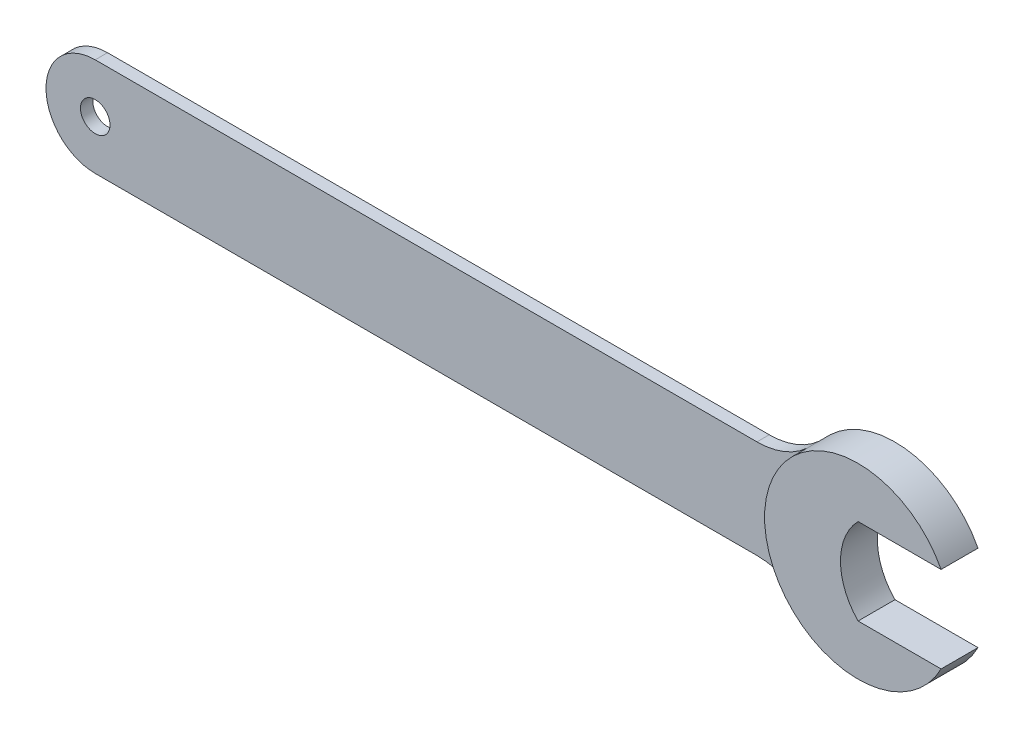
ISO-10303-21;
HEADER;
FILE_DESCRIPTION(('STEP AP214'),'2;1');
FILE_NAME('part.step','',(''),(''),'','','');
FILE_SCHEMA(('AUTOMOTIVE_DESIGN { 1 0 10303 214 1 1 1 1 }'));
ENDSEC;
DATA;
#1=APPLICATION_CONTEXT('core data for automotive mechanical design processes');
#2=APPLICATION_PROTOCOL_DEFINITION('international standard','automotive_design',2000,#1);
#3=PRODUCT_CONTEXT('',#1,'mechanical');
#4=PRODUCT('Part','Part','',(#3));
#5=PRODUCT_RELATED_PRODUCT_CATEGORY('part','',(#4));
#6=PRODUCT_DEFINITION_FORMATION('','',#4);
#7=PRODUCT_DEFINITION_CONTEXT('part definition',#1,'design');
#8=PRODUCT_DEFINITION('design','',#6,#7);
#9=PRODUCT_DEFINITION_SHAPE('','',#8);
#10=(LENGTH_UNIT() NAMED_UNIT(*) SI_UNIT(.MILLI.,.METRE.));
#11=(NAMED_UNIT(*) PLANE_ANGLE_UNIT() SI_UNIT($,.RADIAN.));
#12=(NAMED_UNIT(*) SI_UNIT($,.STERADIAN.) SOLID_ANGLE_UNIT());
#13=UNCERTAINTY_MEASURE_WITH_UNIT(LENGTH_MEASURE(1.E-05),#10,'distance_accuracy_value','');
#14=(GEOMETRIC_REPRESENTATION_CONTEXT(3) GLOBAL_UNCERTAINTY_ASSIGNED_CONTEXT((#13)) GLOBAL_UNIT_ASSIGNED_CONTEXT((#10,
#11,#12)) REPRESENTATION_CONTEXT('',''));
#15=CARTESIAN_POINT('',(0.,0.,0.));
#16=DIRECTION('',(0.,0.,1.));
#17=DIRECTION('',(1.,0.,0.));
#18=AXIS2_PLACEMENT_3D('',#15,#16,#17);
#19=CARTESIAN_POINT('',(315.,20.,0.));
#20=DIRECTION('',(0.,0.,1.));
#21=DIRECTION('',(1.,0.,0.));
#22=AXIS2_PLACEMENT_3D('',#19,#20,#21);
#23=CYLINDRICAL_SURFACE('',#22,38.);
#24=CARTESIAN_POINT('',(315.,20.,-5.));
#25=DIRECTION('',(0.,0.,-1.));
#26=DIRECTION('',(-1.,0.,0.));
#27=AXIS2_PLACEMENT_3D('',#24,#25,#26);
#28=CIRCLE('',#27,38.);
#29=CARTESIAN_POINT('',(348.730549951046,2.5,-5.));
#30=VERTEX_POINT('',#29);
#31=CARTESIAN_POINT('',(348.730549951046,37.5,-5.));
#32=VERTEX_POINT('',#31);
#33=EDGE_CURVE('E149',#30,#32,#28,.T.);
#34=ORIENTED_EDGE('',*,*,#33,.F.);
#35=DIRECTION('',(0.,0.,1.));
#36=VECTOR('',#35,1.);
#37=CARTESIAN_POINT('',(348.730549951046,2.5,0.));
#38=LINE('',#37,#36);
#39=CARTESIAN_POINT('',(348.730549951046,2.5,10.));
#40=VERTEX_POINT('',#39);
#41=EDGE_CURVE('E171',#30,#40,#38,.T.);
#42=ORIENTED_EDGE('',*,*,#41,.T.);
#43=CARTESIAN_POINT('',(315.,20.,10.));
#44=DIRECTION('',(0.,0.,1.));
#45=DIRECTION('',(1.,0.,0.));
#46=AXIS2_PLACEMENT_3D('',#43,#44,#45);
#47=CIRCLE('',#46,38.);
#48=CARTESIAN_POINT('',(348.730549951046,37.5,10.));
#49=VERTEX_POINT('',#48);
#50=EDGE_CURVE('E161',#49,#40,#47,.T.);
#51=ORIENTED_EDGE('',*,*,#50,.F.);
#52=DIRECTION('',(0.,0.,1.));
#53=VECTOR('',#52,1.);
#54=CARTESIAN_POINT('',(348.730549951046,37.5,0.));
#55=LINE('',#54,#53);
#56=EDGE_CURVE('E179',#32,#49,#55,.T.);
#57=ORIENTED_EDGE('',*,*,#56,.F.);
#58=EDGE_LOOP('',(#34,#42,#51,#57));
#59=FACE_BOUND('',#58,.T.);
#60=CARTESIAN_POINT('',(315.,20.,5.));
#61=DIRECTION('',(0.,0.,1.));
#62=DIRECTION('',(1.,0.,0.));
#63=AXIS2_PLACEMENT_3D('',#60,#61,#62);
#64=CIRCLE('',#63,38.);
#65=CARTESIAN_POINT('',(289.245570139499,47.9411764705883,5.));
#66=VERTEX_POINT('',#65);
#67=CARTESIAN_POINT('',(289.245570139499,-7.94117647058826,5.));
#68=VERTEX_POINT('',#67);
#69=EDGE_CURVE('E49',#66,#68,#64,.T.);
#70=ORIENTED_EDGE('',*,*,#69,.T.);
#71=DIRECTION('',(0.,0.,-1.));
#72=VECTOR('',#71,1.);
#73=CARTESIAN_POINT('',(289.245570139499,-7.94117647058827,5.));
#74=LINE('',#73,#72);
#75=CARTESIAN_POINT('',(289.245570139499,-7.94117647058827,0.));
#76=VERTEX_POINT('',#75);
#77=EDGE_CURVE('E130',#68,#76,#74,.T.);
#78=ORIENTED_EDGE('',*,*,#77,.T.);
#79=CARTESIAN_POINT('',(315.,20.,0.));
#80=DIRECTION('',(0.,0.,-1.));
#81=DIRECTION('',(-1.,0.,0.));
#82=AXIS2_PLACEMENT_3D('',#79,#80,#81);
#83=CIRCLE('',#82,38.);
#84=CARTESIAN_POINT('',(289.245570139499,47.9411764705882,0.));
#85=VERTEX_POINT('',#84);
#86=EDGE_CURVE('E11',#76,#85,#83,.T.);
#87=ORIENTED_EDGE('',*,*,#86,.T.);
#88=DIRECTION('',(0.,0.,-1.));
#89=VECTOR('',#88,1.);
#90=CARTESIAN_POINT('',(289.245570139499,47.9411764705883,5.));
#91=LINE('',#90,#89);
#92=EDGE_CURVE('E145',#66,#85,#91,.T.);
#93=ORIENTED_EDGE('',*,*,#92,.F.);
#94=EDGE_LOOP('',(#70,#78,#87,#93));
#95=FACE_BOUND('',#94,.T.);
#96=ADVANCED_FACE('F41',(#59,#95),#23,.T.);
#97=CARTESIAN_POINT('',(315.,40.,5.));
#98=DIRECTION('',(0.,-1.,0.));
#99=DIRECTION('',(0.,0.,-1.));
#100=AXIS2_PLACEMENT_3D('',#97,#98,#99);
#101=PLANE('',#100);
#102=DIRECTION('',(0.,0.,-1.));
#103=VECTOR('',#102,1.);
#104=CARTESIAN_POINT('',(268.913125512788,40.,5.));
#105=LINE('',#104,#103);
#106=CARTESIAN_POINT('',(268.913125512788,40.,5.));
#107=VERTEX_POINT('',#106);
#108=CARTESIAN_POINT('',(268.913125512788,40.,0.));
#109=VERTEX_POINT('',#108);
#110=EDGE_CURVE('E148',#107,#109,#105,.T.);
#111=ORIENTED_EDGE('',*,*,#110,.T.);
#112=DIRECTION('',(-1.,0.,0.));
#113=VECTOR('',#112,1.);
#114=CARTESIAN_POINT('',(315.,40.,0.));
#115=LINE('',#114,#113);
#116=CARTESIAN_POINT('',(0.,40.,0.));
#117=VERTEX_POINT('',#116);
#118=EDGE_CURVE('E192',#109,#117,#115,.T.);
#119=ORIENTED_EDGE('',*,*,#118,.T.);
#120=DIRECTION('',(0.,0.,-1.));
#121=VECTOR('',#120,1.);
#122=CARTESIAN_POINT('',(0.,40.,5.));
#123=LINE('',#122,#121);
#124=CARTESIAN_POINT('',(0.,40.,5.));
#125=VERTEX_POINT('',#124);
#126=EDGE_CURVE('E191',#125,#117,#123,.T.);
#127=ORIENTED_EDGE('',*,*,#126,.F.);
#128=DIRECTION('',(-1.,0.,0.));
#129=VECTOR('',#128,1.);
#130=CARTESIAN_POINT('',(315.,40.,5.));
#131=LINE('',#130,#129);
#132=EDGE_CURVE('E194',#107,#125,#131,.T.);
#133=ORIENTED_EDGE('',*,*,#132,.F.);
#134=EDGE_LOOP('',(#111,#119,#127,#133));
#135=FACE_BOUND('',#134,.T.);
#136=ADVANCED_FACE('F206',(#135),#101,.F.);
#137=CARTESIAN_POINT('',(0.,0.,0.));
#138=DIRECTION('',(0.,0.,1.));
#139=DIRECTION('',(1.,0.,0.));
#140=AXIS2_PLACEMENT_3D('',#137,#138,#139);
#141=PLANE('',#140);
#142=CARTESIAN_POINT('',(0.,20.,0.));
#143=DIRECTION('',(0.,0.,-1.));
#144=DIRECTION('',(-1.,0.,0.));
#145=AXIS2_PLACEMENT_3D('',#142,#143,#144);
#146=CIRCLE('',#145,6.);
#147=CARTESIAN_POINT('',(-6.,20.,0.));
#148=VERTEX_POINT('',#147);
#149=EDGE_CURVE('E139',#148,#148,#146,.T.);
#150=ORIENTED_EDGE('',*,*,#149,.F.);
#151=EDGE_LOOP('',(#150));
#152=FACE_BOUND('',#151,.T.);
#153=ORIENTED_EDGE('',*,*,#86,.F.);
#154=CARTESIAN_POINT('',(268.913125512788,-30.,0.));
#155=DIRECTION('',(0.,0.,1.));
#156=DIRECTION('',(1.,0.,0.));
#157=AXIS2_PLACEMENT_3D('',#154,#155,#156);
#158=CIRCLE('',#157,30.);
#159=CARTESIAN_POINT('',(268.913125512788,0.,0.));
#160=VERTEX_POINT('',#159);
#161=EDGE_CURVE('E118',#76,#160,#158,.T.);
#162=ORIENTED_EDGE('',*,*,#161,.T.);
#163=DIRECTION('',(1.,0.,0.));
#164=VECTOR('',#163,1.);
#165=CARTESIAN_POINT('',(0.,0.,0.));
#166=LINE('',#165,#164);
#167=CARTESIAN_POINT('',(0.,0.,0.));
#168=VERTEX_POINT('',#167);
#169=EDGE_CURVE('E59',#168,#160,#166,.T.);
#170=ORIENTED_EDGE('',*,*,#169,.F.);
#171=CARTESIAN_POINT('',(0.,20.,0.));
#172=DIRECTION('',(0.,0.,1.));
#173=DIRECTION('',(1.,0.,0.));
#174=AXIS2_PLACEMENT_3D('',#171,#172,#173);
#175=CIRCLE('',#174,20.);
#176=EDGE_CURVE('E183',#117,#168,#175,.T.);
#177=ORIENTED_EDGE('',*,*,#176,.F.);
#178=ORIENTED_EDGE('',*,*,#118,.F.);
#179=CARTESIAN_POINT('',(268.913125512788,70.,0.));
#180=DIRECTION('',(0.,0.,1.));
#181=DIRECTION('',(1.,0.,0.));
#182=AXIS2_PLACEMENT_3D('',#179,#180,#181);
#183=CIRCLE('',#182,30.);
#184=EDGE_CURVE('E124',#109,#85,#183,.T.);
#185=ORIENTED_EDGE('',*,*,#184,.T.);
#186=EDGE_LOOP('',(#153,#162,#170,#177,#178,#185));
#187=FACE_BOUND('',#186,.T.);
#188=ADVANCED_FACE('F120',(#152,#187),#141,.F.);
#189=CARTESIAN_POINT('',(0.,0.,5.));
#190=DIRECTION('',(0.,1.,0.));
#191=DIRECTION('',(0.,0.,1.));
#192=AXIS2_PLACEMENT_3D('',#189,#190,#191);
#193=PLANE('',#192);
#194=ORIENTED_EDGE('',*,*,#169,.T.);
#195=DIRECTION('',(0.,0.,-1.));
#196=VECTOR('',#195,1.);
#197=CARTESIAN_POINT('',(268.913125512788,0.,5.));
#198=LINE('',#197,#196);
#199=CARTESIAN_POINT('',(268.913125512788,0.,5.));
#200=VERTEX_POINT('',#199);
#201=EDGE_CURVE('E64',#200,#160,#198,.T.);
#202=ORIENTED_EDGE('',*,*,#201,.F.);
#203=DIRECTION('',(1.,0.,0.));
#204=VECTOR('',#203,1.);
#205=CARTESIAN_POINT('',(0.,0.,5.));
#206=LINE('',#205,#204);
#207=CARTESIAN_POINT('',(0.,0.,5.));
#208=VERTEX_POINT('',#207);
#209=EDGE_CURVE('E188',#208,#200,#206,.T.);
#210=ORIENTED_EDGE('',*,*,#209,.F.);
#211=DIRECTION('',(0.,0.,-1.));
#212=VECTOR('',#211,1.);
#213=CARTESIAN_POINT('',(0.,0.,5.));
#214=LINE('',#213,#212);
#215=EDGE_CURVE('E178',#208,#168,#214,.T.);
#216=ORIENTED_EDGE('',*,*,#215,.T.);
#217=EDGE_LOOP('',(#194,#202,#210,#216));
#218=FACE_BOUND('',#217,.T.);
#219=ADVANCED_FACE('F43',(#218),#193,.F.);
#220=CARTESIAN_POINT('',(0.,0.,5.));
#221=DIRECTION('',(0.,0.,1.));
#222=DIRECTION('',(1.,0.,0.));
#223=AXIS2_PLACEMENT_3D('',#220,#221,#222);
#224=PLANE('',#223);
#225=CARTESIAN_POINT('',(0.,20.,5.));
#226=DIRECTION('',(0.,0.,1.));
#227=DIRECTION('',(1.,0.,0.));
#228=AXIS2_PLACEMENT_3D('',#225,#226,#227);
#229=CIRCLE('',#228,6.);
#230=CARTESIAN_POINT('',(6.,20.,5.));
#231=VERTEX_POINT('',#230);
#232=EDGE_CURVE('E44',#231,#231,#229,.T.);
#233=ORIENTED_EDGE('',*,*,#232,.F.);
#234=EDGE_LOOP('',(#233));
#235=FACE_BOUND('',#234,.T.);
#236=ORIENTED_EDGE('',*,*,#69,.F.);
#237=CARTESIAN_POINT('',(268.913125512788,70.,5.));
#238=DIRECTION('',(0.,0.,1.));
#239=DIRECTION('',(1.,0.,0.));
#240=AXIS2_PLACEMENT_3D('',#237,#238,#239);
#241=CIRCLE('',#240,30.);
#242=EDGE_CURVE('E143',#107,#66,#241,.T.);
#243=ORIENTED_EDGE('',*,*,#242,.F.);
#244=ORIENTED_EDGE('',*,*,#132,.T.);
#245=CARTESIAN_POINT('',(0.,20.,5.));
#246=DIRECTION('',(0.,0.,1.));
#247=DIRECTION('',(1.,0.,0.));
#248=AXIS2_PLACEMENT_3D('',#245,#246,#247);
#249=CIRCLE('',#248,20.);
#250=EDGE_CURVE('E180',#125,#208,#249,.T.);
#251=ORIENTED_EDGE('',*,*,#250,.T.);
#252=ORIENTED_EDGE('',*,*,#209,.T.);
#253=CARTESIAN_POINT('',(268.913125512788,-30.,5.));
#254=DIRECTION('',(0.,0.,1.));
#255=DIRECTION('',(1.,0.,0.));
#256=AXIS2_PLACEMENT_3D('',#253,#254,#255);
#257=CIRCLE('',#256,30.);
#258=EDGE_CURVE('E132',#68,#200,#257,.T.);
#259=ORIENTED_EDGE('',*,*,#258,.F.);
#260=EDGE_LOOP('',(#236,#243,#244,#251,#252,#259));
#261=FACE_BOUND('',#260,.T.);
#262=ADVANCED_FACE('F215',(#235,#261),#224,.T.);
#263=CARTESIAN_POINT('',(0.,20.,0.));
#264=DIRECTION('',(0.,0.,1.));
#265=DIRECTION('',(1.,0.,0.));
#266=AXIS2_PLACEMENT_3D('',#263,#264,#265);
#267=CYLINDRICAL_SURFACE('',#266,20.);
#268=ORIENTED_EDGE('',*,*,#176,.T.);
#269=ORIENTED_EDGE('',*,*,#215,.F.);
#270=ORIENTED_EDGE('',*,*,#250,.F.);
#271=ORIENTED_EDGE('',*,*,#126,.T.);
#272=EDGE_LOOP('',(#268,#269,#270,#271));
#273=FACE_BOUND('',#272,.T.);
#274=ADVANCED_FACE('F201',(#273),#267,.T.);
#275=CARTESIAN_POINT('',(0.,37.5000000000001,0.));
#276=DIRECTION('',(0.,-1.,0.));
#277=DIRECTION('',(1.,0.,0.));
#278=AXIS2_PLACEMENT_3D('',#275,#276,#277);
#279=PLANE('',#278);
#280=ORIENTED_EDGE('',*,*,#56,.T.);
#281=DIRECTION('',(1.,0.,0.));
#282=VECTOR('',#281,1.);
#283=CARTESIAN_POINT('',(348.730549951046,37.5,10.));
#284=LINE('',#283,#282);
#285=CARTESIAN_POINT('',(315.,37.5,10.));
#286=VERTEX_POINT('',#285);
#287=EDGE_CURVE('E172',#286,#49,#284,.T.);
#288=ORIENTED_EDGE('',*,*,#287,.F.);
#289=DIRECTION('',(0.,0.,1.));
#290=VECTOR('',#289,1.);
#291=CARTESIAN_POINT('',(315.,37.5,0.));
#292=LINE('',#291,#290);
#293=CARTESIAN_POINT('',(315.,37.5,-5.));
#294=VERTEX_POINT('',#293);
#295=EDGE_CURVE('E176',#294,#286,#292,.T.);
#296=ORIENTED_EDGE('',*,*,#295,.F.);
#297=DIRECTION('',(-1.,0.,0.));
#298=VECTOR('',#297,1.);
#299=CARTESIAN_POINT('',(348.730549951046,37.5,-5.));
#300=LINE('',#299,#298);
#301=EDGE_CURVE('E153',#32,#294,#300,.T.);
#302=ORIENTED_EDGE('',*,*,#301,.F.);
#303=EDGE_LOOP('',(#280,#288,#296,#302));
#304=FACE_BOUND('',#303,.T.);
#305=ADVANCED_FACE('F222',(#304),#279,.T.);
#306=CARTESIAN_POINT('',(0.,2.5,0.));
#307=DIRECTION('',(0.,-1.,0.));
#308=DIRECTION('',(0.,0.,-1.));
#309=AXIS2_PLACEMENT_3D('',#306,#307,#308);
#310=PLANE('',#309);
#311=DIRECTION('',(0.,0.,1.));
#312=VECTOR('',#311,1.);
#313=CARTESIAN_POINT('',(315.,2.5,0.));
#314=LINE('',#313,#312);
#315=CARTESIAN_POINT('',(315.,2.5,-5.));
#316=VERTEX_POINT('',#315);
#317=CARTESIAN_POINT('',(315.,2.50000000000001,10.));
#318=VERTEX_POINT('',#317);
#319=EDGE_CURVE('E185',#316,#318,#314,.T.);
#320=ORIENTED_EDGE('',*,*,#319,.T.);
#321=DIRECTION('',(-1.,0.,0.));
#322=VECTOR('',#321,1.);
#323=CARTESIAN_POINT('',(348.730549951046,2.5,10.));
#324=LINE('',#323,#322);
#325=EDGE_CURVE('E164',#40,#318,#324,.T.);
#326=ORIENTED_EDGE('',*,*,#325,.F.);
#327=ORIENTED_EDGE('',*,*,#41,.F.);
#328=DIRECTION('',(1.,0.,0.));
#329=VECTOR('',#328,1.);
#330=CARTESIAN_POINT('',(348.730549951046,2.5,-5.));
#331=LINE('',#330,#329);
#332=EDGE_CURVE('E157',#316,#30,#331,.T.);
#333=ORIENTED_EDGE('',*,*,#332,.F.);
#334=EDGE_LOOP('',(#320,#326,#327,#333));
#335=FACE_BOUND('',#334,.T.);
#336=ADVANCED_FACE('F231',(#335),#310,.F.);
#337=CARTESIAN_POINT('',(332.853571071357,20.,0.));
#338=DIRECTION('',(0.,0.,1.));
#339=DIRECTION('',(1.,0.,0.));
#340=AXIS2_PLACEMENT_3D('',#337,#338,#339);
#341=CYLINDRICAL_SURFACE('',#340,25.);
#342=ORIENTED_EDGE('',*,*,#295,.T.);
#343=CARTESIAN_POINT('',(332.853571071357,20.,10.));
#344=DIRECTION('',(0.,0.,-1.));
#345=DIRECTION('',(1.,0.,0.));
#346=AXIS2_PLACEMENT_3D('',#343,#344,#345);
#347=CIRCLE('',#346,25.);
#348=EDGE_CURVE('E169',#318,#286,#347,.T.);
#349=ORIENTED_EDGE('',*,*,#348,.F.);
#350=ORIENTED_EDGE('',*,*,#319,.F.);
#351=CARTESIAN_POINT('',(332.853571071357,20.,-5.));
#352=DIRECTION('',(0.,0.,1.));
#353=DIRECTION('',(-1.,0.,0.));
#354=AXIS2_PLACEMENT_3D('',#351,#352,#353);
#355=CIRCLE('',#354,25.);
#356=EDGE_CURVE('E156',#294,#316,#355,.T.);
#357=ORIENTED_EDGE('',*,*,#356,.F.);
#358=EDGE_LOOP('',(#342,#349,#350,#357));
#359=FACE_BOUND('',#358,.T.);
#360=ADVANCED_FACE('F236',(#359),#341,.F.);
#361=CARTESIAN_POINT('',(315.,20.,10.));
#362=DIRECTION('',(0.,0.,1.));
#363=DIRECTION('',(1.,0.,0.));
#364=AXIS2_PLACEMENT_3D('',#361,#362,#363);
#365=PLANE('',#364);
#366=ORIENTED_EDGE('',*,*,#50,.T.);
#367=ORIENTED_EDGE('',*,*,#325,.T.);
#368=ORIENTED_EDGE('',*,*,#348,.T.);
#369=ORIENTED_EDGE('',*,*,#287,.T.);
#370=EDGE_LOOP('',(#366,#367,#368,#369));
#371=FACE_BOUND('',#370,.T.);
#372=ADVANCED_FACE('F243',(#371),#365,.T.);
#373=CARTESIAN_POINT('',(315.,20.,-5.));
#374=DIRECTION('',(0.,0.,-1.));
#375=DIRECTION('',(-1.,0.,0.));
#376=AXIS2_PLACEMENT_3D('',#373,#374,#375);
#377=PLANE('',#376);
#378=ORIENTED_EDGE('',*,*,#33,.T.);
#379=ORIENTED_EDGE('',*,*,#301,.T.);
#380=ORIENTED_EDGE('',*,*,#356,.T.);
#381=ORIENTED_EDGE('',*,*,#332,.T.);
#382=EDGE_LOOP('',(#378,#379,#380,#381));
#383=FACE_BOUND('',#382,.T.);
#384=ADVANCED_FACE('F250',(#383),#377,.T.);
#385=CARTESIAN_POINT('',(268.913125512788,70.,5.));
#386=DIRECTION('',(0.,0.,-1.));
#387=DIRECTION('',(-1.,0.,0.));
#388=AXIS2_PLACEMENT_3D('',#385,#386,#387);
#389=CYLINDRICAL_SURFACE('',#388,30.);
#390=ORIENTED_EDGE('',*,*,#184,.F.);
#391=ORIENTED_EDGE('',*,*,#110,.F.);
#392=ORIENTED_EDGE('',*,*,#242,.T.);
#393=ORIENTED_EDGE('',*,*,#92,.T.);
#394=EDGE_LOOP('',(#390,#391,#392,#393));
#395=FACE_BOUND('',#394,.T.);
#396=ADVANCED_FACE('F209',(#395),#389,.F.);
#397=CARTESIAN_POINT('',(268.913125512788,-30.,5.));
#398=DIRECTION('',(0.,0.,-1.));
#399=DIRECTION('',(-1.,0.,0.));
#400=AXIS2_PLACEMENT_3D('',#397,#398,#399);
#401=CYLINDRICAL_SURFACE('',#400,30.);
#402=ORIENTED_EDGE('',*,*,#161,.F.);
#403=ORIENTED_EDGE('',*,*,#77,.F.);
#404=ORIENTED_EDGE('',*,*,#258,.T.);
#405=ORIENTED_EDGE('',*,*,#201,.T.);
#406=EDGE_LOOP('',(#402,#403,#404,#405));
#407=FACE_BOUND('',#406,.T.);
#408=ADVANCED_FACE('F135',(#407),#401,.F.);
#409=CARTESIAN_POINT('',(0.,20.,15.));
#410=DIRECTION('',(0.,0.,-1.));
#411=DIRECTION('',(-1.,0.,0.));
#412=AXIS2_PLACEMENT_3D('',#409,#410,#411);
#413=CYLINDRICAL_SURFACE('',#412,6.);
#414=ORIENTED_EDGE('',*,*,#232,.T.);
#415=EDGE_LOOP('',(#414));
#416=FACE_BOUND('',#415,.T.);
#417=ORIENTED_EDGE('',*,*,#149,.T.);
#418=EDGE_LOOP('',(#417));
#419=FACE_BOUND('',#418,.T.);
#420=ADVANCED_FACE('F260',(#416,#419),#413,.F.);
#421=CLOSED_SHELL('',(#96,#136,#188,#219,#262,#274,#305,#336,#360,#372,#384,#396,#408,#420));
#422=MANIFOLD_SOLID_BREP('B2',#421);
#423=ADVANCED_BREP_SHAPE_REPRESENTATION('',(#18,#422),#14);
#424=SHAPE_DEFINITION_REPRESENTATION(#9,#423);
ENDSEC;
END-ISO-10303-21;
